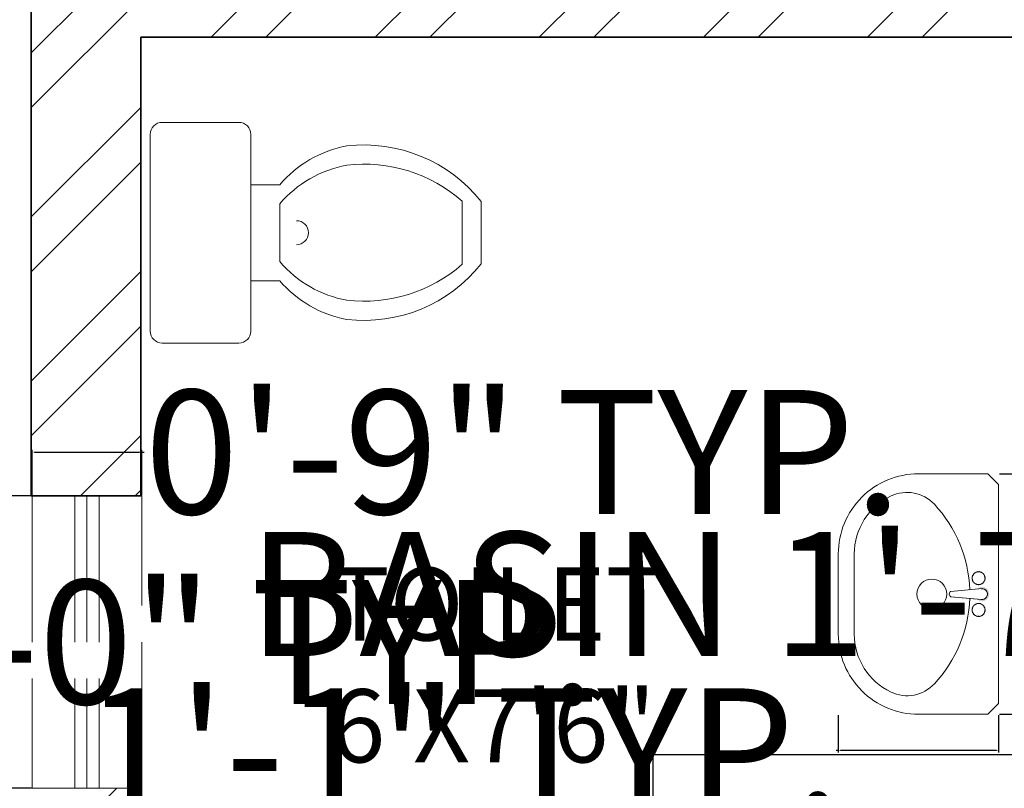
# Model space of a CAD drawing. Units: inches. Extents: x 1812 to 2791, y 2306 to 2959.
# Tile 6 of 8: x 2453 to 2534, y 2793 to 2856. Entities that reach past the tile are written whole.
import ezdxf

# ---------------------------------------------------------------- set-up
doc = ezdxf.new("R2010")
doc.units = ezdxf.units.IN
doc.linetypes.add('ACAD_ISO02W100', pattern=[15, 12, -3])
doc.layers.get('Defpoints').update_dxf_attribs({"lineweight": 50})
for name, color, linetype, lineweight in [('A-ANNO-DIMS', 2, 'Continuous', 18), ('A-AREA-IDEN', 7, 'Continuous', 18), ('A-FLOR-FIXT', 9, 'Continuous', 18), ('A-GLAZ-VENT', 6, 'ACAD_ISO02W100', 13), ('A-WALL-PATT', 8, 'Continuous', 13), ('WALL', 7, 'Continuous', 35)]:
    doc.layers.add(name, color=color, linetype=linetype, lineweight=lineweight)
doc.styles.get("Standard").update_dxf_attribs({"font": 'arial.ttf'})
doc.dimstyles.get("Standard").update_dxf_attribs({"dimtxt": 10.18, "dimasz": 0.18, "dimexe": 0.18, "dimexo": 0.0625, "dimgap": 0.09, "dimtad": 0, "dimtih": 1, "dimtoh": 1, "dimdec": 0, "dimzin": 0, "dimdsep": 46, "dimlunit": 3, "dimtxsty": 'Standard', "dimcen": 0.09, "dimadec": 0, "dimazin": 0, "dimtfac": 1, "dimtdec": 0, "dimtofl": 0, "dimtmove": 0, "dimatfit": 3, "dimfxl": 1, "dimtolj": 1, "dimtzin": 0, "dimarcsym": 0})

# ---------------------------------------------------------------- blocks, each defined once
blk = doc.blocks.new('A$C2AC94788')
for p, q in [((0.0250000842625013, 0.6899999873276103), (0.4350000842623559, 0.6899999873276103)), ((8.42619556e-08, 0.5049999873299384), (8.42619556e-08, 0.664999987326155)), ((0.4600000842619921, 0.664999987326155), (0.4600000842619921, 0.5049999873299384)), ((0.4350000842623559, 0.4799999873284833), (0.0250000842625013, 0.4799999873284833)), ((0.1300000842620648, 0.4799999873284833), (0.1300000842620648, 0.4199999873308116)), ((0.3300000842618829, 0.4199999873308116), (0.3300000842618829, 0.4799999873284833)), ((0.1700000842620284, 0.4199999873308116), (0.2900000842619192, 0.4199999873308116)), ((0.1640625266463758, 0.0391832446184708), (0.2959376418775719, 0.0391832446184708)), ((0.2290625266468851, 0.0391832446184708), (0.2300046331329213, 0.0391832446184708)), ((0.2309376418770626, 0.0391832446184708), (0.2299955353910263, 0.0391832446184708)), ((0.1650000842619192, -1.26747182e-08), (0.2950000842620284, -1.26747182e-08))]:
    blk.add_line(p, q)
for centre, radius, start, end in [((0.0250000842625013, 0.664999987326155), 0.025, 90, 180), ((0.4350000842623559, 0.664999987326155), 0.025, 0, 90), ((0.0250000842625013, 0.5049999873299384), 0.025, 180, 270), ((0.4350000842623559, 0.5049999873299384), 0.025, 270, 0), ((0.2874442183401697, 0.2355819240110577), 0.2424843859558644, 130.488541879527, 169.445013547103), ((0.3274442183401334, 0.2355819240110577), 0.2424843859558644, 130.488541879527, 169.445013547103), ((0.1325559501838143, 0.2355819240110577), 0.2424843859558745, 10.55498645289699, 49.51145812047296), ((0.1725559501837779, 0.2355819240110577), 0.2424843859558745, 10.55498645289699, 49.51145812047296), ((0.2300000842624286, 0.3849999873273191), 0.025, 180, 0), ((0.3600593119572294, 0.2447691737834247), 0.3129857136460789, 173.5368801771597, 231.4482773914608), ((0.4000593119571932, 0.2447691737834248), 0.3129857136460972, 173.5368801771598, 221.0603827222079), ((0.0999408565667182, 0.2447691737834248), 0.3129857136460789, 308.5517226085392, 6.463119822840183), ((0.0599408565667545, 0.2447691737834248), 0.3129857136460896, 318.9396172777922, 6.463119822840183)]:
    blk.add_arc(centre, radius, start, end)
blk = doc.blocks.new('s_46')
at = {"ltscale": 600}
h = blk.add_hatch(color=256, dxfattribs=at)
edge = h.paths.add_edge_path()
edge.add_line((13.45184378023259, 62.04360352296498), (14.15927104179718, 54.09782096462731))
edge.add_ellipse((4.212458010588306, 52.31250418393756), major_axis=(-10.10576298371302, 2.5e-15), ratio=1, start_angle=540, end_angle=550.1754626554052, ccw=False)
edge.add_arc((4.212458010588306, 52.31250418393756), 10.10576298371302, 270, 360, ccw=False)
edge.add_line((4.212458010588306, 42.20674120020703), (4.212458010588306, 41.28018079043977))
edge.add_line((4.212458010588306, 41.28018079040339), (11.85106942148559, 41.28018079040339))
edge.add_arc((4.212458010588306, 52.31250418393756), 13.41866400745597, 664.6981342835142, 766.4847699121552)
h.paths.add_polyline_path([(4.212458010588306, 41.28018079040339), (-3.426153400272596, 41.28018079040339, 0.152566653256377), (4.212458010588306, 38.8938401764608)])
h.paths.add_polyline_path([(11.85106942144921, 41.28018079040339), (4.212458010588306, 41.28018079040339), (4.212458010588306, 38.8938401764608, 0.1525666532563772)])
h.paths.add_polyline_path([(-5.734355020395014, 54.09782096461277), (-5.026927758881356, 62.04360352296498, 0.4758332592079194), (-3.426153400272596, 41.28018079040339), (4.212458010588306, 41.28018079040339), (4.212458010588306, 42.20674120020703, -0.4672400657637396)])
for p, q in [((-5.893304973142221, 52.31250418385025), (-0.714987907151226, 110.4750654234667)), ((-5.893304973142221, 52.31250418385025), (-0.714987907151226, 110.4750654234667)), ((9.139903928502463, 110.475065423554), (14.15927104174625, 54.09782096461277)), ((14.31822099431883, 52.31250418385025), (9.139903928502463, 110.475065423554)), ((14.15927104174625, 54.09782096461277), (14.31822099431883, 52.31250418385025))]:
    blk.add_line(p, q, dxfattribs=at)
blk.add_lwpolyline([(-220.7875419894117, 171.2801807903452, -0.4142135623730951), (-70.7875419894117, 321.2801807903452), (79.2124580105883, 321.2801807904325, -0.4142135623730951), (229.2124580105883, 171.2801807904325), (229.2124580105883, 41.28018079040339), (209.2124580107047, 21.2801807904325), (-200.7875419893535, 21.28018079034518), (-220.7875419894117, 41.28018079040339)], format="xyb", close=True, dxfattribs=at)
blk.add_lwpolyline([(12.26164246437838, 75.41187665969483, 0.1816379869150311), (172.1859176590806, 141.5383421540609, 0.3263505073803008), (187.6570333366981, 222.6589125997853, 0.2898144196813102), (79.21245801076293, 291.2801807904325), (-70.78754198923707, 291.2801807903452, 0.2898144196813102), (-179.2321173155214, 222.658912599698, 0.3263505073803008), (-163.7610016377293, 141.5383421540609, 0.1816379869150315), (-3.836726442852523, 75.41187665960751)], format="xyb", dxfattribs=at)
for points in [[(-16.83803374727722, 67.43055756771354), (-17.02338931558188, 67.50428807432763), (-17.22058725368697, 67.56961317334208), (-17.42189012444578, 67.6347039079701), (-17.61956049106084, 67.70773132116301), (-17.80586091603618, 67.79686645595939), (-17.97305396257434, 67.91028035557245), (-18.11578784312587, 68.05326030802098), (-18.23825336818117, 68.21955858168076), (-18.34702699835179, 68.40004368982045), (-18.44868519355077, 68.58558414605795), (-18.54980441438965, 68.76704846357461), (-18.65696112113073, 68.9353051558137), (-18.77673177386168, 69.08122273621848), (-18.91569283319404, 69.19566971814493), (-19.07841429975815, 69.27267628890695), (-19.26144033775199, 69.31891933156292), (-19.45930865121772, 69.34423740339116), (-19.66655694507062, 69.35846906132065), (-19.87772292352747, 69.37145286262967), (-20.08734429115429, 69.39302736415993), (-20.2899587523425, 69.43303112310241), (-20.48010401183274, 69.50130269664805), (-20.65391131333308, 69.60429419830325), (-20.81388605764368, 69.73491196823306), (-20.96412718523061, 69.8826759030926), (-21.10873363655992, 70.03710589953698), (-21.25180435174844, 70.18772185422131), (-21.39743827126222, 70.3240436638007), (-21.54973433539272, 70.43559122501756), (-21.71279148443137, 70.5118844343524), (-21.88955151231494, 70.54600451889564), (-22.07832762773614, 70.54527802669325), (-22.27627589285839, 70.52059283622657), (-22.4805523698451, 70.48283682571491), (-22.68831312085968, 70.44289787355228), (-22.89671420806553, 70.41166385821998), (-23.10291169380071, 70.40002265802468), (-23.30406164005399, 70.41886215136037), (-23.49802141042892, 70.4753938675276), (-23.68545357254334, 70.56212393892929), (-23.86772199510597, 70.66788214896224), (-24.04619054717477, 70.78149828102323), (-24.22222309763311, 70.89180211850908), (-24.39718351518968, 70.98762344472925), (-24.57243566872785, 71.05779204316786), (-24.74934342730558, 71.09113769704709), (-24.92903553397628, 71.08022740500746), (-25.11170022917213, 71.03257702605333), (-25.2972906283685, 70.95943963443278), (-25.48575984616764, 70.8720683044812), (-25.67706099752104, 70.7817161102721), (-25.87114719772944, 70.69963612605352), (-26.0679715613951, 70.63708142607356), (-26.26748720381875, 70.60530508466763), (-26.46941223740578, 70.61182491958607), (-26.67252476507565, 70.64921772302478), (-26.87536788737634, 70.70632503094384), (-27.07648470485583, 70.77198837930337), (-27.27441831788747, 70.8350493038015), (-27.46771182701923, 70.88434934031102), (-27.6549083327991, 70.90873002487933), (-27.83455093560042, 70.8970328932919), (-28.00620139669627, 70.84190539614065), (-28.17349611973623, 70.75121864315588), (-28.34109016874572, 70.63664965887438), (-28.51363860827405, 70.50987546765828), (-28.69579650234664, 70.38257309404435), (-28.89221891516354, 70.26641956248204), (-29.10756091127405, 70.17309189750813), (-29.3464775547036, 70.11426712348475), (-29.61160253512208, 70.0940409177856), (-29.89748404390411, 70.0861835690448), (-30.19664889771957, 70.05688401864609), (-30.50162391323829, 69.9723312081478), (-30.80493590747938, 69.79871407902101), (-31.09911169676343, 69.50222157256212), (-31.37667809793493, 69.0490426304168), (-31.63016192783834, 68.40536619405611), (-32.32050594605971, 68.4500712644367), (-32.84873653826071, 68.3918758847285), (-33.24226493795868, 68.25193804170704), (-33.52850237919483, 68.0514157223224), (-33.73486009566113, 67.8114669136994), (-33.88874932087492, 67.5532496026135), (-34.01758128887741, 67.29792177610216), (-34.14876723336056, 67.06664142102818), (-34.30371923936764, 66.87550954936887), (-34.47985279804561, 66.72039927294827), (-34.66858425136889, 66.59212672835565), (-34.86132994201034, 66.48150805244222), (-35.04950621211901, 66.37935938188457), (-35.22452940384392, 66.27649685335928), (-35.37781585985795, 66.16373660371755), (-35.50078192248475, 66.03189476963598), (-35.58785390376579, 65.87432967920904), (-35.64549799636007, 65.69456842611542), (-35.68319036299363, 65.49868029527715), (-35.7104071660433, 65.2927345718781), (-35.73662456823513, 65.08280054092756), (-35.77131873212056, 64.87494748734753), (-35.82396582007641, 64.67524469623459), (-35.90404199482873, 64.48976145259803), (-36.01774371694773, 64.3227640100813), (-36.15814863995183, 64.17130649695173), (-36.31505471485434, 64.0306400101108), (-36.47825989319244, 63.89601564637269), (-36.63756212632871, 63.76268450255157), (-36.78275936545106, 63.62589767554891), (-36.90364956192207, 63.48090626226621), (-36.99003066710429, 63.32296135951764), (-37.03518227743916, 63.14869254492805), (-37.04631056915969, 62.96024331927765), (-37.03410336375237, 62.7611356638954), (-37.00924848217983, 62.55489156045951), (-36.98243374592858, 62.34503299021162), (-36.96434697631048, 62.13508193491725), (-36.96567599463743, 61.92856037581805), (-36.99710862222128, 61.72899029450491), (-37.06570762058254, 61.53896291530691), (-37.16403551277472, 61.35734643402975), (-37.28102976223454, 61.18207828939194), (-37.40562783187488, 61.0110959201993), (-37.52676718513249, 60.84233676508302), (-37.63338528544409, 60.67373826284892), (-37.7144195958972, 60.50323785204091), (-37.75880757992855, 60.32877297155209), (-37.75920177751686, 60.14875038337777), (-37.72311503690435, 59.96345414296957), (-37.66177528270055, 59.77363762940512), (-37.58641044021351, 59.58005422132555), (-37.5082484340528, 59.38345729780849), (-37.43851718935184, 59.18460023758234), (-37.38844463089481, 58.98423641963745), (-37.36925868364051, 58.78311922278953), (-37.38844463089481, 58.58200202594161), (-37.43851718935184, 58.38163820799673), (-37.5082484340528, 58.18278114777058), (-37.58641044021351, 57.98618422425352), (-37.66177528287517, 57.79260081626126), (-37.72311503690435, 57.6027843026095), (-37.75920177751686, 57.4174880622013), (-37.75880757992855, 57.23746547402697), (-37.7144195958972, 57.06300059353816), (-37.63338528544409, 56.89250018273014), (-37.52676718530711, 56.72390168049606), (-37.40562783187488, 56.55514252537978), (-37.28102976223454, 56.38416015618713), (-37.16403551277472, 56.20889201154932), (-37.06570762058254, 56.02727553035947), (-36.99710862222128, 55.83724815107416), (-36.96567599463743, 55.63767806976102), (-36.96434697631048, 55.43115651066182), (-36.98243374592858, 55.22120545536745), (-37.00924848217983, 55.01134688520687), (-37.03410336375237, 54.80510278168367), (-37.04631056933431, 54.60599512638873), (-37.03518227743916, 54.41754590065102), (-36.99003066710429, 54.24327708606142), (-36.90364956192207, 54.08533218331285), (-36.78275936545106, 53.94034077003016), (-36.63756212632871, 53.80355394302751), (-36.47825989319244, 53.67022279920639), (-36.31505471502896, 53.53559843546827), (-36.15814863995183, 53.39493194862734), (-36.01774371712236, 53.24347443549777), (-35.90404199482873, 53.07647699298104), (-35.82396582007641, 52.89099374934449), (-35.77131873212056, 52.69129095823155), (-35.73662456823513, 52.48343790465151), (-35.71040716621792, 52.27350387370098), (-35.68319036299363, 52.06755815021461), (-35.64549799653469, 51.87167001946363), (-35.58785390376579, 51.69190876637003), (-35.50078192248475, 51.53434367594309), (-35.3778353385278, 51.40284301002975), (-35.22468523163116, 51.29247093791491), (-35.05003213009331, 51.19609060572111), (-34.86257656256203, 51.10656515930895), (-34.67101905716118, 51.01675774488831), (-34.48406014236389, 50.91953150840708), (-34.31040034646867, 50.80774959607516), (-34.15874019777402, 50.67427515375311), (-34.03505195630714, 50.51453334218241), (-33.93439480883535, 50.3341973797942), (-33.84909967368003, 50.14150249981321), (-33.77149746881332, 49.94468393520219), (-33.69391911290586, 49.75197691909852), (-33.60869552427903, 49.57161668455228), (-33.50815762107959, 49.41183846470085), (-33.38463632145431, 49.28087749250699), (-33.23284944484476, 49.18408373402781), (-33.05706241185544, 49.11526608630083), (-32.86392754490953, 49.06534817945794), (-32.66009716555709, 49.02525364354369), (-32.45222359569743, 48.98590610860265), (-32.24695915722987, 48.93822920459206), (-32.05095617187908, 48.87314656155649), (-31.870866961719, 48.78158180962782), (-31.71133844077122, 48.65761859554914), (-31.5689958925941, 48.50798063381808), (-31.43845919286832, 48.34255165536887), (-31.31434821744915, 48.17121539139771), (-31.19128284219187, 48.00385557310073), (-31.06388294277713, 47.85035593167413), (-30.92676839523483, 47.72060019822674), (-30.77455907507101, 47.62447210386745), (-30.60346923320321, 47.56846716045401), (-30.41609062027419, 47.54552800310193), (-30.21660936163971, 47.54520904741366), (-30.00921158283018, 47.55706470907898), (-29.79808340937598, 47.570649403875), (-29.58741096680751, 47.57551754757878), (-29.38138038065517, 47.56122355579281), (-29.18417777627474, 47.51732184420689), (-28.99883273948217, 47.43692629240103), (-28.8237486963626, 47.32738863455597), (-28.65617253311211, 47.19962006882997), (-28.49335113610141, 47.06453179311938), (-28.33253139152657, 46.9330350055825), (-28.1709601857583, 46.81604090429027), (-28.00588440499268, 46.72446068713907), (-27.83455093577504, 46.66920555219985), (-27.6549083327991, 46.65750842061243), (-27.46771182701923, 46.68188910518074), (-27.27441831788747, 46.73118914177758), (-27.07648470485583, 46.7942500662757), (-26.87536788755096, 46.85991341454792), (-26.67252476525027, 46.91702072246698), (-26.4694122375804, 46.95441352590569), (-26.26748720399337, 46.96093336082412), (-26.06797156156972, 46.9291570194182), (-25.87114719772944, 46.86660231943824), (-25.67706099769566, 46.78452233530697), (-25.48575984616764, 46.69417014101054), (-25.2972906283685, 46.60679881105898), (-25.11170022934675, 46.53366141943843), (-24.92903553397628, 46.4860110404843), (-24.74934342730558, 46.47510074844467), (-24.57243566890247, 46.50844640232389), (-24.39718351536431, 46.57861500076251), (-24.22222309780773, 46.67443632698268), (-24.0461905473494, 46.78474016446853), (-23.86772199528059, 46.89835629652953), (-23.68545357254334, 47.00411450656247), (-23.49802141060354, 47.09084457796416), (-23.30406164022861, 47.14737629413138), (-23.10291169380071, 47.16621578746708), (-22.89671420806553, 47.15457458727178), (-22.68831312085968, 47.12334057193948), (-22.4805523698451, 47.08340161977685), (-22.27627589285839, 47.04564560926519), (-22.07832762791077, 47.02096041871118), (-21.88955151248956, 47.02023392650881), (-21.71279148443137, 47.05435401113937), (-21.54973433539272, 47.1306472204742), (-21.39743827126222, 47.24219478160375), (-21.25180435174844, 47.37851659118314), (-21.10873363655992, 47.52913254586746), (-20.96412718540523, 47.68356254231185), (-20.81388605764368, 47.83132647717138), (-20.65391131333308, 47.9619442471012), (-20.48010401200736, 48.0649357488437), (-20.28995875251712, 48.13320732230204), (-20.08734429115429, 48.17321108133183), (-19.87772292352747, 48.1947855828621), (-19.66655694507062, 48.2077693840838), (-19.45930865139235, 48.2220010421006), (-19.26144033775199, 48.24731911384152), (-19.07841429993277, 48.29356215667212), (-18.91569283319404, 48.37056872743414), (-18.77673177403631, 48.48501570936059), (-18.65696112113073, 48.63093328976538), (-18.54980441456428, 48.79918998200446), (-18.44868519372539, 48.98065429960843), (-18.34702699835179, 49.16619475575862), (-18.2382533683558, 49.34667986398562), (-18.11578784312587, 49.5129781376454), (-17.97305396274896, 49.6559580900066), (-17.8058609162108, 49.76937198961969), (-17.61956049106084, 49.85850712450337), (-17.4218901246204, 49.93153453769628), (-17.22058725368697, 49.996625272237), (-17.02338931558188, 50.06195037133875), (-16.83803374727722, 50.13568087795284), (-16.67225798609434, 50.22598783511785), (-16.53379946883069, 50.34104228604701), (-16.42766593385022, 50.48645191569812), (-16.34794632298872, 50.65757097714231), (-16.28599987912457, 50.84719036528259), (-16.23318584513618, 51.04810097528389), (-16.18086346407654, 51.25309370196191), (-16.12039197882404, 51.45495944039431), (-16.04313063243171, 51.64648908557137), (-15.94043866742868, 51.82047353248345), (-15.8067031877581, 51.97190354572376), (-15.64842273970134, 52.10456936812261), (-15.47512373042991, 52.22446111202589), (-15.29633256676607, 52.33756888969219), (-15.12157565605594, 52.44988281364204), (-14.96037940529641, 52.567392996134), (-14.82227022130973, 52.69608954960131), (-14.71677451161667, 52.84196258638985), (-14.6501372611965, 53.00919824198354), (-14.61547776852967, 53.19476674450561), (-14.60263391025364, 53.3938343450427), (-14.60144356318051, 53.60156729485606), (-14.60174460412236, 53.81313184503233), (-14.59337490954203, 54.02369424700736), (-14.566172356077, 54.22842075169319), (-14.50997482053935, 54.42247761052567), (-14.41809999983525, 54.6024088327249), (-14.29778487142175, 54.77026946117985), (-14.1597462335485, 54.92949229647638), (-14.01470088359201, 55.08351013963693), (-13.87336561962729, 55.23575579150929), (-13.7464572393801, 55.38966205302859), (-13.64469254092546, 55.54866172495531), (-13.5787883218145, 55.71618760822457), (-13.55583441938506, 55.89474125843844), (-13.56841282837558, 56.08309925056528), (-13.60547858278733, 56.27910691397847), (-13.65598671662155, 56.48060957840062), (-13.70889226370491, 56.68545257346704), (-13.7531502583879, 56.89148122872575), (-13.7777157346718, 57.09654087381204), (-13.77154372638324, 57.29847683827393), (-13.72730239736847, 57.49560352915432), (-13.65251243085367, 57.68811166286468), (-13.55840763938613, 57.8766610333987), (-13.45622183586238, 58.06191143448813), (-13.35718883317895, 58.24452266012667), (-13.27254244388314, 58.42515450413339), (-13.2135164810461, 58.60446676041465), (-13.19134475721512, 58.78311922278953), (-13.2135164810461, 58.96177168516442), (-13.27254244388314, 59.14108394144569), (-13.35718883317895, 59.3217157854524), (-13.45622183586238, 59.50432701109093), (-13.55840763938613, 59.68957741218037), (-13.65251243085367, 59.87812678271438), (-13.72730239736847, 60.07063491642475), (-13.77154372638324, 60.26776160730515), (-13.7777157346718, 60.46969757176703), (-13.7531502583879, 60.67475721685332), (-13.70889226370491, 60.88078587211203), (-13.65598671662155, 61.08562886717845), (-13.60547858278733, 61.2871315316006), (-13.56841282837558, 61.48313919501379), (-13.55583441938506, 61.67149718714063), (-13.5787883218145, 61.8500508373545), (-13.64469254092546, 62.01757672062377), (-13.7464572393801, 62.17657639255048), (-13.87336561962729, 62.33048265406978), (-14.01470088359201, 62.48272830594214), (-14.15974623337388, 62.63674614910269), (-14.29778487142175, 62.79596898448653), (-14.41809999983525, 62.96382961285416), (-14.50997482053935, 63.14376083514071), (-14.566172356077, 63.33781769388588), (-14.59337490936741, 63.5425441985717), (-14.60174460412236, 63.75310660054674), (-14.60144356318051, 63.96467115081032), (-14.60263391025364, 64.17240410053635), (-14.61547776835505, 64.37147170116077), (-14.65013726102188, 64.55704020359553), (-14.71677451144205, 64.7242758591892), (-14.82227022130973, 64.87014889597776), (-14.96037940529641, 64.99884544944507), (-15.12157565605594, 65.11635563193704), (-15.29633256676607, 65.22866955588688), (-15.47512373042991, 65.3417773336405), (-15.64842273970134, 65.46166907745646), (-15.8067031877581, 65.59433489985531), (-15.94043866742868, 65.74576491309563), (-16.04313063225709, 65.9197493600077), (-16.12039197882404, 66.11127900527208), (-16.18086346407654, 66.31314474370447), (-16.23318584513618, 66.5181374703825), (-16.28599987912457, 66.71904808029649), (-16.34794632298872, 66.90866746843676), (-16.42766593385022, 67.07978652988095), (-16.53379946883069, 67.22519615953206), (-16.67225798609434, 67.34025061046123)], [(22.08090273779817, 61.08562886709115), (22.03039460413856, 61.2871315315133), (21.99332884972682, 61.48313919501379), (21.9807504407363, 61.67149718705331), (22.00370434316574, 61.85005083726719), (22.06960856210208, 62.01757672053645), (22.17137326073134, 62.17657639246318), (22.29828164080391, 62.33048265398247), (22.43961690476863, 62.48272830585483), (22.58466225472512, 62.63674614901538), (22.72270089277299, 62.79596898439923), (22.84301602118649, 62.96382961276686), (22.93489084189059, 63.1437608350534), (22.99108837742824, 63.33781769379857), (23.01829093071865, 63.5425441985717), (23.0266606254736, 63.75310660045943), (23.02635958453175, 63.96467115072301), (23.02754993160488, 64.17240410053635), (23.04039378970629, 64.37147170107346), (23.07505328237312, 64.55704020350822), (23.14169053279329, 64.72427585910191), (23.24718624266097, 64.87014889589045), (23.38529542664764, 64.99884544935776), (23.54649167740717, 65.11635563193704), (23.7212485881173, 65.22866955579956), (23.90003975178115, 65.34177733355318), (24.07333876105258, 65.46166907736915), (24.23161920910934, 65.594334899768), (24.36535468877992, 65.74576491300832), (24.46804665360833, 65.9197493600077), (24.54530800017528, 66.11127900518477), (24.60577948542777, 66.31314474361714), (24.65810186648742, 66.51813747029519), (24.71091590047581, 66.71904808020918), (24.77286234433996, 66.90866746834945), (24.85258195520146, 67.07978652979364), (24.95871549018193, 67.22519615953206), (25.09717400744558, 67.34025061046123), (25.26294976862846, 67.43055756771354), (25.44830533693312, 67.50428807432763), (25.64550327503821, 67.56961317334208), (25.84680614579702, 67.6347039079701), (26.04447651241208, 67.70773132116301), (26.23077693756204, 67.79686645595939), (26.3979699841002, 67.91028035557245), (26.54070386447711, 68.05326030802098), (26.66316938970704, 68.21955858168076), (26.77194301970303, 68.40004368982045), (26.87360121507663, 68.58558414605795), (26.97472043591552, 68.76704846357461), (27.08187714248197, 68.9353051558137), (27.20164779538754, 69.08122273621848), (27.34060885454528, 69.19566971814493), (27.50333032128401, 69.27267628890695), (27.68635635910323, 69.31891933165025), (27.88422467274358, 69.34423740347847), (28.09147296642186, 69.35846906140794), (28.30263894487871, 69.37145286262967), (28.51226031250553, 69.39302736424725), (28.71487477386836, 69.43303112318972), (28.90502003318398, 69.50130269673537), (29.07882733468432, 69.60429419839056), (29.23880207899492, 69.73491196832038), (29.38904320658185, 69.88267590317992), (29.53364965791116, 70.0371058996243), (29.67672037309967, 70.18772185430862), (29.82235429261346, 70.324043663888), (29.97465035674395, 70.43559122501756), (30.1377075057826, 70.51188443443971), (30.31446753366618, 70.54600451898295), (30.50324364908738, 70.54527802678058), (30.70119191420963, 70.52059283622657), (30.90546839119634, 70.48283682571491), (31.11322914221091, 70.4428978736396), (31.32163022941677, 70.41166385830729), (31.52782771515195, 70.400022658112), (31.72897766157985, 70.41886215144768), (31.92293743178016, 70.4753938675276), (32.11036959389458, 70.56212393892929), (32.29263801663183, 70.66788214896224), (32.47110656870063, 70.78149828102323), (32.64713911898434, 70.89180211850908), (32.82209953654092, 70.98762344481656), (32.99735169025371, 71.05779204316786), (33.17425944865681, 71.09113769704709), (33.35395155532751, 71.08022740500746), (33.53661625069799, 71.03257702605333), (33.72220664971974, 70.9594396345201), (33.91067586751888, 70.8720683044812), (34.1019770190469, 70.7817161102721), (34.29606321908068, 70.69963612605352), (34.49288758292096, 70.63708142616088), (34.69240322534461, 70.60530508466763), (34.89432825893164, 70.61182491958607), (35.09744078660151, 70.64921772302478), (35.3002839089022, 70.70632503103116), (35.50140072620707, 70.77198837930337), (35.6993343392387, 70.8350493038015), (35.89262784837047, 70.88434934039833), (36.07982435415034, 70.90873002487933), (36.25946695695166, 70.8970328932919), (36.43111741804751, 70.84190539614065), (36.59841214108747, 70.75121864315588), (36.76600619009696, 70.63664965887438), (36.93855462962529, 70.50987546765828), (37.12071252369788, 70.38257309404435), (37.3171349366894, 70.26641956248204), (37.53247693262529, 70.17309189750813), (37.77139357605483, 70.11426712348475), (38.03651855647331, 70.0940409177856), (38.32240006525535, 70.0861835690448), (38.62156491907081, 70.05688401864609), (38.92653993476415, 69.9723312081478), (39.22985192883061, 69.79871407893368), (39.52402771811467, 69.50222157256212), (39.80159411928616, 69.0490426304168), (40.05507794918957, 68.4053661939688), (40.74542196741094, 68.4500712644367), (41.27365255961194, 68.3918758846412), (41.66718095948453, 68.25193804161972), (41.95341840054607, 68.0514157223224), (42.15977611701236, 67.8114669136121), (42.31366534240078, 67.5532496025262), (42.44249731022864, 67.29792177601485), (42.57368325471179, 67.06664142094087), (42.72863526071887, 66.87550954936887), (42.90476881939684, 66.72039927286096), (43.09350027272012, 66.59212672826834), (43.28624596336157, 66.48150805235491), (43.47442223347025, 66.37935938179726), (43.64944542536977, 66.27649685335928), (43.80273188138381, 66.16373660371755), (43.92569794383598, 66.03189476963598), (44.01276992511703, 65.87432967912173), (44.0704140177113, 65.69456842602813), (44.10810638434486, 65.49868029527715), (44.13532318739453, 65.2927345718781), (44.16154058958636, 65.08280054084025), (44.19623475347179, 64.87494748726021), (44.24888184142765, 64.67524469614727), (44.32895801617997, 64.48976145251072), (44.44265973829897, 64.32276400999397), (44.58306466130307, 64.17130649695173), (44.73997073620558, 64.03064001002348), (44.90317591454368, 63.89601564628538), (45.06247814767994, 63.76268450246425), (45.20767538680229, 63.6258976754616), (45.3285655832733, 63.4809062621789), (45.41494668845553, 63.32296135943034), (45.46009829879039, 63.14869254484074), (45.47122659051092, 62.96024331919034), (45.45901938492898, 62.76113566380809), (45.43416450353106, 62.5548915603722), (45.40734976727981, 62.34503299021162), (45.38926299766171, 62.13508193482994), (45.39059201598866, 61.92856037573074), (45.42202464357251, 61.7289902944176), (45.49062364193377, 61.53896291521959), (45.58895153412595, 61.35734643394243), (45.70594578341115, 61.18207828939194), (45.83054385322611, 61.01109592011198), (45.95168320648371, 60.84233676508302), (46.05830130679533, 60.67373826276162), (46.13933561724843, 60.50323785204091), (46.18372360127978, 60.32877297146479), (46.1841177988681, 60.14875038329046), (46.14803105825558, 59.96345414296957), (46.08669130405178, 59.77363762931782), (46.01132646156474, 59.58005422123824), (45.93316445540404, 59.38345729772118), (45.86343321070308, 59.18460023749503), (45.81336065224604, 58.98423641955014), (45.79417470499175, 58.78311922270222), (45.81336065224604, 58.58200202585431), (45.86343321070308, 58.38163820790942), (45.93316445540404, 58.18278114777058), (46.01132646156474, 57.98618422416621), (46.08669130405178, 57.79260081617394), (46.14803105808095, 57.6027843025222), (46.1841177988681, 57.4174880622013), (46.18372360127978, 57.23746547393966), (46.13933561724843, 57.06300059345085), (46.05830130679533, 56.89250018273014), (45.95168320648371, 56.72390168040874), (45.83054385322611, 56.55514252529247), (45.70594578341115, 56.38416015609982), (45.58895153412595, 56.20889201154932), (45.49062364193377, 56.02727553027216), (45.42202464339789, 55.83724815107416), (45.39059201598866, 55.63767806976102), (45.38926299766171, 55.43115651066182), (45.40734976727981, 55.22120545528014), (45.43416450335644, 55.01134688511957), (45.45901938492898, 54.80510278159636), (45.47122659051092, 54.60599512630142), (45.46009829879039, 54.41754590056371), (45.41494668845553, 54.24327708597411), (45.32856558309868, 54.08533218322554), (45.20767538662767, 53.94034076994285), (45.06247814750532, 53.8035539429402), (44.90317591454368, 53.67022279920639), (44.73997073620558, 53.53559843538096), (44.58306466130307, 53.39493194854004), (44.44265973829897, 53.24347443541046), (44.32895801617997, 53.07647699298104), (44.24888184125302, 52.89099374934449), (44.19623475329717, 52.69129095823155), (44.16154058958636, 52.48343790465151), (44.13532318739453, 52.27350387361366), (44.10810638434486, 52.06755815021461), (44.0704140177113, 51.87167001946363), (44.01276992511703, 51.69190876628272), (43.92569794366136, 51.53434367585578), (43.80275135970442, 51.40284301002975), (43.64960125280776, 51.29247093791491), (43.47494815144455, 51.1960906056338), (43.28749258373863, 51.10656515922165), (43.09593507851241, 51.01675774480099), (42.90897616371512, 50.91953150840708), (42.73531636764528, 50.80774959598784), (42.58365621895063, 50.67427515375311), (42.45996797765838, 50.51453334218241), (42.35931083018658, 50.3341973797942), (42.27401569485664, 50.14150249981321), (42.19641349016455, 49.94468393520219), (42.1188351342571, 49.75197691909852), (42.03361154545564, 49.57161668455228), (41.9330736422562, 49.41183846461354), (41.80955234280554, 49.28087749250699), (41.65776546602137, 49.1840837339405), (41.48197843320668, 49.11526608630083), (41.28884356608614, 49.06534817945794), (41.0850131867337, 49.02525364354369), (40.87713961687405, 48.98590610851534), (40.67187517840648, 48.93822920459206), (40.47587219323031, 48.87314656155649), (40.29578298289561, 48.78158180962782), (40.13625446194782, 48.65761859554914), (39.99391191377072, 48.50798063373076), (39.86337521404493, 48.34255165528157), (39.73926423862577, 48.17121539139771), (39.61619886336848, 48.00385557310073), (39.48879896395374, 47.85035593167413), (39.35168441641144, 47.72060019813944), (39.19947509624762, 47.62447210378013), (39.02838525455445, 47.56846716045401), (38.8410066414508, 47.54552800310193), (38.64152538281633, 47.54520904732635), (38.43412760400679, 47.55706470907898), (38.22299943072721, 47.570649403875), (38.01232698798413, 47.57551754757878), (37.80629640183179, 47.56122355579281), (37.60909379745135, 47.51732184420689), (37.42374876065878, 47.43692629240103), (37.24866471753922, 47.32738863455597), (37.08108855428873, 47.19962006882997), (36.91826715727803, 47.06453179311938), (36.75744741270319, 46.9330350056698), (36.59587620693492, 46.81604090429027), (36.4308004261693, 46.72446068713907), (36.25946695695166, 46.66920555228716), (36.07982435397571, 46.65750842061243), (35.89262784837047, 46.68188910518074), (35.6993343392387, 46.73118914177758), (35.50140072620707, 46.7942500662757), (35.30028390872758, 46.85991341454792), (35.09744078642689, 46.91702072246698), (34.89432825875701, 46.954413525993), (34.69240322516998, 46.96093336082412), (34.49288758274633, 46.9291570194182), (34.29606321908068, 46.86660231943824), (34.10197701887228, 46.78452233530697), (33.91067586734425, 46.69417014109785), (33.72220664971974, 46.60679881105898), (33.53661625052337, 46.53366141943843), (33.35395155515289, 46.4860110404843), (33.17425944865681, 46.47510074844467), (32.99735169007909, 46.5084464024112), (32.82209953654092, 46.57861500076251), (32.64713911898434, 46.67443632707), (32.47110656852601, 46.78474016446853), (32.2926380164572, 46.89835629661684), (32.11036959389458, 47.00411450664979), (31.92293743178016, 47.09084457805147), (31.72897766140522, 47.14737629413138), (31.52782771497732, 47.16621578746708), (31.32163022941677, 47.15457458727178), (31.11322914203629, 47.12334057193948), (30.90546839102171, 47.08340161986416), (30.70119191420963, 47.0456456093525), (30.50324364908738, 47.02096041879849), (30.31446753366618, 47.02023392659611), (30.1377075057826, 47.05435401113937), (29.97465035674395, 47.13064722056151), (29.82235429261346, 47.24219478169106), (29.67672037309967, 47.37851659127045), (29.53364965791116, 47.52913254595478), (29.38904320658185, 47.68356254239916), (29.2388020788203, 47.8313264772587), (29.0788273345097, 47.96194424718851), (28.90502003318398, 48.06493574893102), (28.71487477369374, 48.13320732238935), (28.51226031250553, 48.17321108133183), (28.30263894487871, 48.19478558294941), (28.09147296642186, 48.20776938417111), (27.88422467256896, 48.22200104218791), (27.68635635892861, 48.24731911392882), (27.50333032110939, 48.29356215667212), (27.34060885454528, 48.37056872743414), (27.20164779521292, 48.48501570936059), (27.08187714248197, 48.63093328976538), (26.97472043574089, 48.79918998200446), (26.87360121490201, 48.98065429960843), (26.77194301952841, 49.16619475575862), (26.66316938953241, 49.34667986398562), (26.54070386447711, 49.51297813755809), (26.39796998392558, 49.6559580900066), (26.23077693738742, 49.76937198961969), (26.04447651223745, 49.85850712450337), (25.84680614579702, 49.93153453769628), (25.64550327486359, 49.996625272237), (25.44830533675849, 50.06195037133875), (25.26294976862846, 50.13568087795284), (25.09717400727095, 50.22598783520516), (24.95871549018193, 50.34104228604701), (24.85258195520146, 50.48645191561082), (24.77286234416534, 50.657570977055), (24.71091590030119, 50.84719036519527), (24.65810186648742, 51.04810097519657), (24.60577948542777, 51.2530937018746), (24.54530800017528, 51.45495944030699), (24.46804665360833, 51.64648908548406), (24.36535468877992, 51.82047353239614), (24.23161920910934, 51.97190354572376), (24.07333876105258, 52.1045693680353), (23.90003975160653, 52.22446111193858), (23.7212485881173, 52.33756888960488), (23.54649167740717, 52.44988281355472), (23.38529542647302, 52.56739299604669), (23.24718624266097, 52.696089549514), (23.14169053279329, 52.84196258630254), (23.07505328237312, 53.00919824189623), (23.04039378970629, 53.1947667444183), (23.02754993160488, 53.39383434495539), (23.02635958453175, 53.60156729476876), (23.02666062529898, 53.81313184503233), (23.01829093071865, 54.02369424692006), (22.99108837725362, 54.22842075169319), (22.93489084171597, 54.42247761043836), (22.84301602101186, 54.6024088327249), (22.72270089277299, 54.77026946109254), (22.58466225472512, 54.92949229638907), (22.43961690476863, 55.08351013963693), (22.29828164080391, 55.23575579150929), (22.17137326073134, 55.38966205294127), (22.06960856210208, 55.548661724868), (22.00370434316574, 55.71618760813726), (21.9807504407363, 55.89474125843844), (21.99332884972682, 56.08309925047797), (22.03039460413856, 56.27910691389115), (22.08090273779817, 56.48060957840062), (22.13380828505615, 56.68545257346704), (22.17806627973914, 56.89148122872575), (22.20263175602304, 57.09654087381204), (22.19645974773448, 57.29847683827393), (22.15221841871971, 57.49560352915432), (22.07742845220491, 57.68811166286468), (21.98332366073737, 57.87666103331139), (21.88113785721362, 58.06191143448813), (21.78210485453019, 58.24452266012667), (21.69745846523438, 58.42515450413339), (21.63843250239734, 58.60446676032734), (21.61626077856636, 58.78311922270222), (21.63843250239734, 58.96177168507711), (21.69745846523438, 59.14108394135837), (21.78210485453019, 59.32171578536508), (21.88113785721362, 59.50432701100362), (21.98332366073737, 59.68957741209306), (22.07742845220491, 59.87812678262708), (22.15221841871971, 60.07063491633743), (22.19645974773448, 60.26776160721784), (22.20263175602304, 60.46969757167971), (22.17806627973914, 60.67475721676601), (22.13380828505615, 60.88078587202471)]]:
    blk.add_lwpolyline(points, close=True, dxfattribs=at)
blk.add_circle((4.212458010588306, 146.2801807904034), 28, dxfattribs=at)
for centre, radius, start, end in [((4.212458010588306, 108.2109541267855), 5.422722861947412, 24.67830004152974, 155.3216999584702), ((4.212458010588306, 52.31250418393756), 10.10576298371233, 169.8245373479931, 0)]:
    blk.add_arc(centre, radius, start, end, dxfattribs=at)
for centre, major_axis, ratio, start_param, end_param in [((4.212458010762929, 110.475065423554), (-4.927445917859709, 1.2e-15), 0.6410240960233505, 3.141592653589793, 6.283185307179586), ((4.212458010588306, 52.31250418393756), (-10.10576298371302, 2.5e-15), 1, 6.105589980929039, 9.602373287019926)]:
    blk.add_ellipse(centre, major_axis=major_axis, ratio=ratio, start_param=start_param, end_param=end_param, dxfattribs=at)
blk = doc.blocks.new('VENT-24x9')
for p, q in [((3.499863851171994, 23.99973038050894), (3.499863851171994, -0.0002696194910641)), ((4.499863851171994, 23.99973038050894), (4.499863851171994, -0.0002696194910641)), ((5.499863851171994, 23.99973038050894), (5.499863851171994, -0.0002696194910641))]:
    blk.add_line(p, q)
blk.add_lwpolyline([(-0.0001361485951747, -0.0002696194910641), (8.999863851404825, -0.0002696194910641), (8.999863851171995, 23.99973038050894), (-0.0001361488280054, 23.99973038050894)], close=True)
blk = doc.blocks.new('*D48')
at = {"layer": 'A-ANNO-DIMS', "color": 0, "lineweight": -2, "transparency": 16777216}
for p, q in [((2454.200753859796, 2816.957881357629), (2450.483253859797, 2816.957881357629)), ((2450.663253859797, 2816.777881357629), (2450.663253859797, 2810.245514372636)), ((2450.663253859797, 2793.137881357629), (2450.663253859797, 2799.670248342622)), ((2454.200753859796, 2792.957881357629), (2450.483253859797, 2792.957881357629))]:
    blk.add_line(p, q, dxfattribs=at)
at = {"layer": 'A-ANNO-DIMS', "color": 0, "transparency": 16777216}
for points in [[(2450.633253859797, 2816.777881357629), (2450.693253859797, 2816.777881357629), (2450.663253859797, 2816.957881357629)], [(2450.633253859797, 2793.137881357629), (2450.693253859797, 2793.137881357629), (2450.663253859797, 2792.957881357629)]]:
    blk.add_solid(points, dxfattribs=at)
at = {"layer": 'Defpoints', "color": 0, "transparency": 16777216}
for p in [(2450.663253859797, 2816.957881357629), (2454.263253859796, 2816.957881357629), (2454.263253859796, 2792.957881357629)]:
    blk.add_point(p, dxfattribs=at)
at = {"layer": 'A-ANNO-DIMS', "color": 0, "transparency": 16777216, "insert": (2450.663253859797, 2804.957881357628), "char_height": 10.18, "attachment_point": 5}
blk.add_mtext('\\A1;VENT 2\'-0" TYP.', dxfattribs=at)
blk = doc.blocks.new('*D49')
at = {"layer": 'A-ANNO-DIMS', "color": 0, "lineweight": -2, "transparency": 16777216}
for p, q in [((2454.263253859795, 2817.020381357628), (2454.263253859795, 2820.737881357628)), ((2454.443253859795, 2820.557881357628), (2463.083253860028, 2820.557881357628)), ((2463.263253860028, 2817.020381357628), (2463.263253860028, 2820.737881357628)), ((2463.263253860028, 2820.557881357628), (2463.443253860028, 2820.557881357628))]:
    blk.add_line(p, q, dxfattribs=at)
at = {"layer": 'A-ANNO-DIMS', "color": 0, "transparency": 16777216}
for points in [[(2454.443253859795, 2820.587881357628), (2454.443253859795, 2820.527881357628), (2454.263253859795, 2820.557881357628)], [(2463.083253860028, 2820.587881357628), (2463.083253860028, 2820.527881357628), (2463.263253860028, 2820.557881357628)]]:
    blk.add_solid(points, dxfattribs=at)
at = {"layer": 'Defpoints', "color": 0, "transparency": 16777216}
for p in [(2463.263253860028, 2820.557881357628), (2454.263253859795, 2816.957881357629), (2463.263253860028, 2816.957881357629)]:
    blk.add_point(p, dxfattribs=at)
at = {"layer": 'A-ANNO-DIMS', "color": 0, "transparency": 16777216, "insert": (2494.559338443929, 2820.557881357628), "char_height": 10.18, "attachment_point": 5}
blk.add_mtext('\\A1;0\'-9" TYP.', dxfattribs=at)
blk = doc.blocks.new('*D58')
at = {"layer": 'A-ANNO-DIMS', "color": 0, "lineweight": -2, "transparency": 16777216}
for p, q in [((2533.666907414658, 2818.774380578327), (2536.746255119824, 2818.774380578327)), ((2536.566255119824, 2818.594380578328), (2536.566255119824, 2814.255156531551)), ((2536.566255119824, 2799.20872921056), (2536.566255119824, 2803.547953257336)), ((2533.666907414658, 2799.02872921056), (2536.746255119824, 2799.02872921056))]:
    blk.add_line(p, q, dxfattribs=at)
at = {"layer": 'A-ANNO-DIMS', "color": 0, "transparency": 16777216}
for points in [[(2536.536255119824, 2818.594380578328), (2536.596255119824, 2818.594380578328), (2536.566255119824, 2818.774380578327)], [(2536.536255119824, 2799.20872921056), (2536.596255119824, 2799.20872921056), (2536.566255119824, 2799.02872921056)]]:
    blk.add_solid(points, dxfattribs=at)
at = {"layer": 'Defpoints', "color": 0, "transparency": 16777216}
for p in [(2533.604407414657, 2818.774380578327), (2533.604407414657, 2799.02872921056), (2536.566255119824, 2799.02872921056)]:
    blk.add_point(p, dxfattribs=at)
at = {"layer": 'A-ANNO-DIMS', "color": 0, "transparency": 16777216, "insert": (2536.566255119824, 2808.901554894443), "char_height": 10.18, "attachment_point": 5}
blk.add_mtext('\\A1;BASIN 1\'-7 1/2" TYP.', dxfattribs=at)
blk = doc.blocks.new('*D59')
at = {"layer": 'A-ANNO-DIMS', "color": 0, "lineweight": -2, "transparency": 16777216}
for p, q in [((2520.440639836141, 2798.966229210559), (2520.440639836141, 2795.886881505393)), ((2533.604407414657, 2798.966229210559), (2533.604407414657, 2795.886881505393)), ((2520.440639836141, 2796.066881505393), (2520.260639836141, 2796.066881505393)), ((2533.424407414657, 2796.066881505393), (2520.620639836141, 2796.066881505393))]:
    blk.add_line(p, q, dxfattribs=at)
at = {"layer": 'A-ANNO-DIMS', "color": 0, "transparency": 16777216}
for points in [[(2520.620639836141, 2796.096881505393), (2520.620639836141, 2796.036881505393), (2520.440639836141, 2796.066881505393)], [(2533.424407414657, 2796.096881505393), (2533.424407414657, 2796.036881505393), (2533.604407414657, 2796.066881505393)]]:
    blk.add_solid(points, dxfattribs=at)
at = {"layer": 'Defpoints', "color": 0, "transparency": 16777216}
for p in [(2520.440639836141, 2799.028729210559), (2533.604407414657, 2799.028729210559), (2520.440639836141, 2796.066881505393)]:
    blk.add_point(p, dxfattribs=at)
at = {"layer": 'A-ANNO-DIMS', "color": 0, "transparency": 16777216, "insert": (2489.623695770657, 2796.066881505393), "char_height": 10.18, "attachment_point": 5}
blk.add_mtext('\\A1;1\'-1" TYP.', dxfattribs=at)
blk = doc.blocks.new('*D60')
at = {"layer": 'A-ANNO-DIMS', "color": 0, "lineweight": -2, "transparency": 16777216}
for p, q in [((2505.177694196558, 2790.74953182163), (2500.089565400664, 2790.74953182163)), ((2500.269565400663, 2790.56953182163), (2500.269565400663, 2779.537842838497)), ((2500.269565400663, 2757.792006515665), (2500.269565400663, 2768.823695498797)), ((2505.177694196558, 2757.612006515665), (2500.089565400664, 2757.612006515665))]:
    blk.add_line(p, q, dxfattribs=at)
at = {"layer": 'A-ANNO-DIMS', "color": 0, "transparency": 16777216}
for points in [[(2500.239565400664, 2790.56953182163), (2500.299565400664, 2790.56953182163), (2500.269565400663, 2790.74953182163)], [(2500.239565400664, 2757.792006515665), (2500.299565400664, 2757.792006515665), (2500.269565400663, 2757.612006515665)]]:
    blk.add_solid(points, dxfattribs=at)
at = {"layer": 'Defpoints', "color": 0, "transparency": 16777216}
for p in [(2500.269565400663, 2790.74953182163), (2505.240194196558, 2790.74953182163), (2505.240194196558, 2757.612006515665)]:
    blk.add_point(p, dxfattribs=at)
at = {"layer": 'A-ANNO-DIMS', "color": 0, "transparency": 16777216, "insert": (2500.269565400663, 2774.180769168646), "char_height": 10.18, "attachment_point": 5}
blk.add_mtext('\\A1;DOOR 2\'-9" TYP.', dxfattribs=at)
blk = doc.blocks.new('*D61')
at = {"layer": 'A-ANNO-DIMS', "color": 0, "lineweight": -2, "transparency": 16777216}
for p, q in [((2505.240194196556, 2790.812031821629), (2505.240194196556, 2795.900160617524)), ((2505.420194196557, 2795.720160617524), (2535.060194196564, 2795.720160617524)), ((2535.240194196564, 2790.812031821629), (2535.240194196564, 2795.900160617524)), ((2535.240194196564, 2795.720160617524), (2535.420194196563, 2795.720160617524))]:
    blk.add_line(p, q, dxfattribs=at)
at = {"layer": 'A-ANNO-DIMS', "color": 0, "transparency": 16777216}
for points in [[(2505.420194196557, 2795.750160617524), (2505.420194196557, 2795.690160617523), (2505.240194196556, 2795.720160617524)], [(2535.060194196564, 2795.750160617524), (2535.060194196564, 2795.690160617523), (2535.240194196564, 2795.720160617524)]]:
    blk.add_solid(points, dxfattribs=at)
at = {"layer": 'Defpoints', "color": 0, "transparency": 16777216}
for p in [(2535.240194196564, 2795.720160617524), (2505.240194196556, 2790.749531821629), (2535.240194196564, 2790.749531821629)]:
    blk.add_point(p, dxfattribs=at)
at = {"layer": 'A-ANNO-DIMS', "color": 0, "transparency": 16777216, "insert": (2566.623079599019, 2795.720160617524), "char_height": 10.18, "attachment_point": 5}
blk.add_mtext('\\A1;2\'-6" TYP.', dxfattribs=at)

msp = doc.modelspace()

# ---------------------------------------------------------------- hatches: boundary and pattern name
at = {"layer": 'A-WALL-PATT'}
h = msp.add_hatch(dxfattribs=at)
h.set_pattern_fill('ANSI32', color=256)
h.set_pattern_definition([(45, (563.8057507655523, 20.01067828916757), (-6.735192090801865, 6.735192090801866), []), (45, (568.2958807655523, 20.01067828916757), (-6.735192090801865, 6.735192090801866), [])])
h.paths.add_polyline_path([(2694.192292649419, 2437.613622010101), (2683.499516441466, 2437.6136220101), (2683.499516441466, 2788.569354872347), (2685.192292649419, 2788.569354872347), (2685.192292649419, 2821.63505754476), (2685.125860943268, 2869.374403893766), (2685.125860943268, 2821.63505754476), (2694.192292649419, 2821.63505754476)])
h.paths.add_polyline_path([(2587.192292649419, 2446.613622010096), (2463.19229264942, 2446.613622010089), (2463.19229264942, 2473.613622010101), (2515.608214234135, 2473.613622010101), (2515.608214234135, 2477.6136220101), (2463.19229264942, 2477.6136220101), (2463.19229264942, 2610.6136220101), (2523.737487215154, 2610.613622010101), (2523.737487215154, 2614.613622010101), (2463.19229264942, 2614.6136220101), (2463.19229264942, 2654.536135698824), (2454.192292649419, 2654.536135698824), (2454.192292649419, 2437.613622010101), (2587.192292649419, 2437.613622010101)])
h.paths.add_polyline_path([(2683.499516441466, 2446.6136220101), (2676.19229264942, 2446.6136220101), (2676.192292649419, 2437.6136220101), (2683.499516441466, 2437.613622010101)])
h.paths.add_polyline_path([(2463.192292649419, 2760.6136220101), (2505.192292649419, 2760.6136220101), (2505.192292649419, 2764.6136220101), (2463.192292649419, 2764.6136220101), (2463.192292649419, 2792.952050683902), (2454.192292649419, 2792.952050683902), (2454.192292649419, 2702.536135698824), (2463.016486285651, 2702.536135698824), (2463.016486285651, 2702.649195550402)])
h.paths.add_polyline_path([(2539.192292649419, 2858.613622010101), (2463.192292649419, 2858.6136220101), (2463.192292649419, 2876.345134993912), (2454.192292649419, 2876.345134993912), (2454.19229264942, 2816.957881357627), (2463.192292649419, 2816.957881357627), (2463.192292649419, 2854.6136220101), (2535.192292649419, 2854.613622010101), (2535.192292649419, 2760.6136220101), (2539.192292649419, 2760.6136220101)])
h.paths.add_polyline_path([(2683.499516441466, 2917.613622010101), (2454.192292649419, 2917.613622010101), (2454.192292649419, 2900.372408669677), (2463.192292649419, 2900.372408669677), (2463.192292649419, 2908.6136220101), (2683.499516441466, 2908.613622010101)])
h.paths.add_polyline_path([(2694.192292649419, 2917.613622010101), (2683.499516441466, 2917.613622010101), (2683.499516441466, 2908.613622010101), (2685.192292649419, 2908.613622010101), (2685.192292649419, 2869.63505754476), (2694.192292649419, 2869.63505754476)])

# ---------------------------------------------------------------- linework, layer by layer
at = {"layer": 'WALL'}
for p, q in [((2454.19229264942, 2816.952050683903), (2454.192292649419, 2876.345134993912)), ((2463.19229264942, 2854.6136220101), (2535.192292649419, 2854.613622010101)), ((2463.192292649419, 2816.952050683903), (2463.192292649419, 2854.613622010099)), ((2463.192292649419, 2816.952050683902), (2454.192292649419, 2816.952050683903))]:
    msp.add_line(p, q, dxfattribs=at)

# ---------------------------------------------------------------- block references
at = {"layer": 'A-FLOR-FIXT', "rotation": 90}
for name, p, xscale, yscale, zscale in [('A$C2AC94788', (2491.118410759568, 2829.508417668881), 39.375, 39.375, 39.375), ('s_46', (2534.538165261166, 2809.086394288395), -0.0438792252617072, 0.0438792252617072, 0.0438792252617072)]:
    msp.add_blockref(name, p, dxfattribs=dict(at, xscale=xscale, yscale=yscale, zscale=zscale))
at = {"layer": 'A-GLAZ-VENT'}
msp.add_blockref('VENT-24x9', (2454.263390008623, 2792.958150977119), dxfattribs=at)

# ---------------------------------------------------------------- texts
at = {"layer": 'A-AREA-IDEN', "insert": (2478.708152100318, 2811.086175900971), "char_height": 6, "attachment_point": 1}
msp.add_mtext_dynamic_manual_height_columns('TOILET\\P6\'X7\'6"', width=184.43951469184, gutter_width=12.5, heights=[0], dxfattribs=at)

# ---------------------------------------------------------------- dimensions: what is measured, and where the dimension line sits
at = {"layer": 'A-ANNO-DIMS'}
for base, p1, p2, angle, text, picture, middle in [((2536.566255119824, 2799.02872921056), (2533.604407414657, 2818.774380578327), (2533.604407414657, 2799.028729210559), 270, 'BASIN <> TYP.', '*D58', (2536.566255119824, 2808.901554894443)), ((2450.663253859797, 2816.957881357629), (2454.263253859795, 2792.957881357628), (2454.263253859795, 2816.957881357629), 90, 'VENT <> TYP.', '*D48', (2450.663253859797, 2804.957881357628)), ((2520.440639836141, 2796.066881505393), (2533.604407414657, 2799.028729210559), (2520.440639836141, 2799.028729210559), 180, '<> TYP.', '*D59', (2489.623695770657, 2796.066881505393)), ((2500.269565400663, 2790.74953182163), (2505.240194196556, 2757.612006515664), (2505.240194196556, 2790.749531821629), 90, 'DOOR <> TYP.', '*D60', (2500.269565400663, 2774.180769168646))]:
    dim = msp.add_linear_dim(base=base, p1=p1, p2=p2, angle=angle, text=text, dimstyle='Standard', override={"dimdec": 1, "dimlfac": 1, "dimrnd": 0, "dimzin": 1, "dimdsep": 46, "dimlunit": 4, "dimfrac": 2}, dxfattribs=at)
    dim.commit()
    dim.dimension.update_dxf_attribs({"geometry": picture, "text_midpoint": middle})
for base, p1, p2, picture, middle in [((2463.263253860028, 2820.557881357628), (2454.263253859795, 2816.957881357629), (2463.263253860028, 2816.957881357629), '*D49', (2494.559338443929, 2820.557881357628)), ((2535.240194196564, 2795.720160617524), (2505.240194196556, 2790.749531821629), (2535.240194196564, 2790.749531821629), '*D61', (2566.623079599019, 2795.720160617524))]:
    dim = msp.add_linear_dim(base=base, p1=p1, p2=p2, text='<> TYP.', dimstyle='Standard', override={"dimdec": 1, "dimlfac": 1, "dimrnd": 0, "dimzin": 1, "dimdsep": 46, "dimlunit": 4, "dimfrac": 2}, dxfattribs=at)
    dim.commit()
    dim.dimension.update_dxf_attribs({"geometry": picture, "text_midpoint": middle})

doc.saveas('drawing.dxf')
